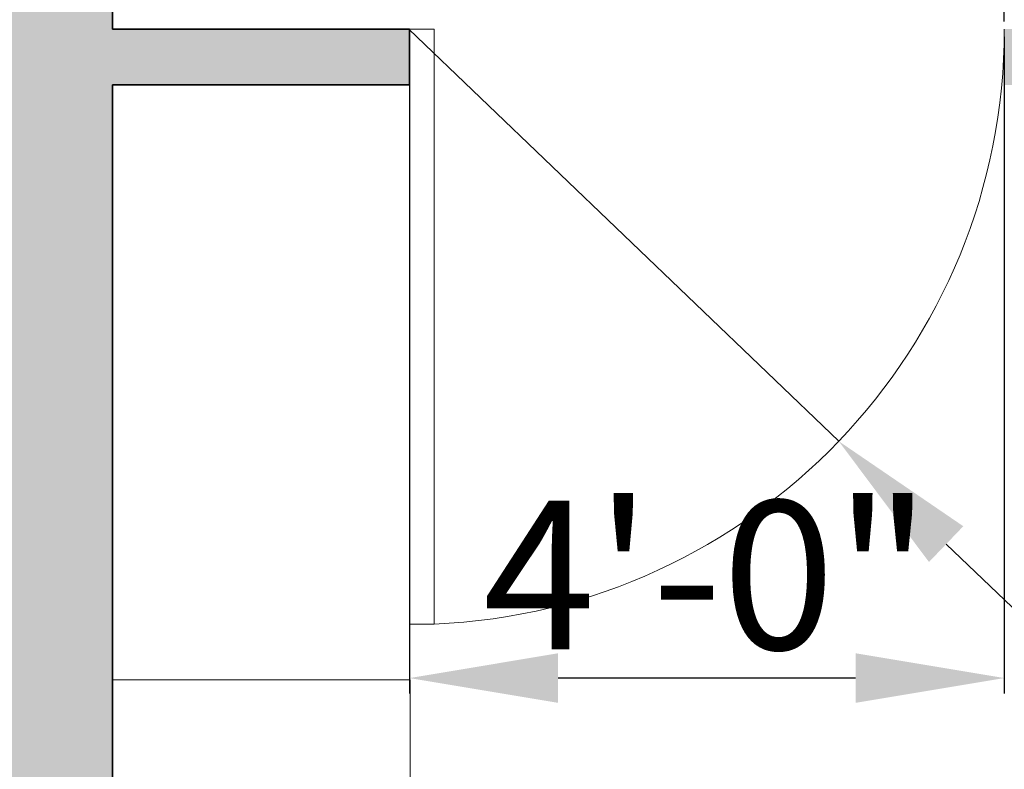
# Model space of a CAD drawing. Units: inches. Extents: x 2083 to 3317, y 1141 to 2115.
# Tile 113 of 256: x 2864 to 2944, y 1361 to 1422. Entities that reach past the tile are written whole.
import ezdxf

# ---------------------------------------------------------------- set-up
doc = ezdxf.new("R2010")
doc.units = ezdxf.units.IN
for name, color, linetype, lineweight in [('A-ANNO-DIMS', 2, 'Continuous', 18), ('A-DOOR', 4, 'Continuous', 18), ('A-FLOR-CASE', 8, 'Continuous', 18), ('A-WALL', 7, 'Continuous', 35)]:
    doc.layers.add(name, color=color, linetype=linetype, lineweight=lineweight)
doc.layers.add('A-WALL-PATT', color=251, linetype='Continuous', lineweight=13, true_color=0x636466)
doc.styles.get("Standard").update_dxf_attribs({"font": 'arial.ttf'})
doc.dimstyles.new('ISO-25', dxfattribs={"dimtxt": 12, "dimasz": 12, "dimexe": 1.25, "dimexo": 0.625, "dimtad": 1, "dimlunit": 3, "dimtxsty": 'Standard', "dimcen": 2.5, "dimadec": 0, "dimazin": 0, "dimtfac": 1, "dimtmove": 0, "dimatfit": 3, "dimfxl": 1, "dimarcsym": 0})

# ---------------------------------------------------------------- blocks, each defined once
blk = doc.blocks.new('CASEWORK-96X24')
for q in [(0, 0), (24, 96)]:
    blk.add_line((0, 96), q)
blk = doc.blocks.new('*D48')
at = {"layer": 'A-ANNO-DIMS', "color": 0, "lineweight": -2, "transparency": 16777216}
for p, q in [((2871.96, 1421.386), (2871.96, 1474.361)), ((2943.91, 1421.386), (2943.91, 1474.361)), ((2883.96, 1473.111), (2931.91, 1473.111))]:
    blk.add_line(p, q, dxfattribs=at)
at = {"layer": 'A-ANNO-DIMS', "color": 0, "transparency": 16777216}
for points in [[(2883.96, 1475.111), (2883.96, 1471.111), (2871.96, 1473.111)], [(2931.91, 1475.111), (2931.91, 1471.111), (2943.91, 1473.111)]]:
    blk.add_solid(points, dxfattribs=at)
at = {"layer": 'Defpoints', "color": 0, "transparency": 16777216}
for p in [(2943.91, 1473.111), (2871.96, 1420.761), (2943.91, 1420.761)]:
    blk.add_point(p, dxfattribs=at)
at = {"layer": 'A-ANNO-DIMS', "color": 0, "transparency": 16777216, "insert": (2907.935, 1479.863), "char_height": 12, "attachment_point": 5}
blk.add_mtext('6\'-0"', dxfattribs=at)
blk = doc.blocks.new('*D59')
at = {"layer": 'A-ANNO-DIMS', "color": 0, "lineweight": -2, "transparency": 16777216}
for p, q in [((2895.91, 1420.136), (2895.91, 1367.161)), ((2943.91, 1420.136), (2943.91, 1367.161)), ((2931.91, 1368.411), (2907.91, 1368.411))]:
    blk.add_line(p, q, dxfattribs=at)
at = {"layer": 'A-ANNO-DIMS', "color": 0, "transparency": 16777216}
for points in [[(2907.91, 1370.411), (2907.91, 1366.411), (2895.91, 1368.411)], [(2931.91, 1370.411), (2931.91, 1366.411), (2943.91, 1368.411)]]:
    blk.add_solid(points, dxfattribs=at)
at = {"layer": 'Defpoints', "color": 0, "transparency": 16777216}
for p in [(2895.91, 1420.761), (2943.91, 1420.761), (2895.91, 1368.411)]:
    blk.add_point(p, dxfattribs=at)
at = {"layer": 'A-ANNO-DIMS', "color": 0, "transparency": 16777216, "insert": (2919.91, 1375.163), "char_height": 12, "attachment_point": 5}
blk.add_mtext('4\'-0"', dxfattribs=at)
blk = doc.blocks.new('*D73')
at = {"layer": 'A-ANNO-DIMS', "color": 0, "lineweight": -2, "transparency": 16777216}
for p, q in [((2895.865, 1420.763), (2930.553, 1387.52)), ((2980.105, 1340.032), (2939.217, 1379.217))]:
    blk.add_line(p, q, dxfattribs=at)
at = {"layer": 'A-ANNO-DIMS', "color": 0, "transparency": 16777216}
blk.add_solid([(2940.601, 1380.661), (2937.833, 1377.773), (2930.553, 1387.52)], dxfattribs=at)
at = {"layer": 'Defpoints', "color": 0, "transparency": 16777216}
for p in [(2895.865, 1420.763), (2930.553, 1387.52)]:
    blk.add_point(p, dxfattribs=at)
at = {"layer": 'A-ANNO-DIMS', "color": 0, "transparency": 16777216, "insert": (2968.665, 1360.348), "char_height": 12, "attachment_point": 5, "rotation": 316.21871}
blk.add_mtext('R4\'-0"', dxfattribs=at)

msp = doc.modelspace()

# ---------------------------------------------------------------- hatches: boundary and pattern name
at = {"layer": 'A-WALL-PATT'}
h = msp.add_hatch(color=256, dxfattribs=at)
h.dxf.hatch_style = 1
h.paths.add_polyline_path([(3126.96, 2020.761), (2748.96, 2020.761), (2604.96, 2020.761), (2226.96, 2020.761), (2226.96, 1702.761), (2466.96, 1702.761), (2466.96, 1582.761), (2418.96, 1582.761), (2418.96, 1477.761), (2226.96, 1477.761), (2226.96, 1263.261), (2544.96, 1263.261), (2544.96, 1411.761), (2604.96, 1411.761), (2685.96, 1411.761), (2685.96, 1420.761), (2604.96, 1420.761), (2604.96, 1573.761), (2604.96, 1702.761), (2604.96, 2011.761), (2748.96, 2011.761), (2748.96, 1702.761), (2862.96, 1702.761), (2862.96, 1621.761), (2871.96, 1621.761), (2871.96, 1702.761), (2883.96, 1702.761), (2883.96, 1706.939, -0.026459), (2883.96, 1711.761), (2757.96, 1711.761), (2757.96, 1807.761), (2787.96, 1807.761), (2787.96, 1812.261), (2757.96, 1812.261), (2757.96, 2011.761), (2877.96, 2011.761), (2877.96, 1812.261), (2847.96, 1812.261), (2847.96, 1807.761), (2889.836, 1807.761), (2889.836, 1812.261), (2882.46, 1812.261), (2882.46, 2011.761), (3117.96, 2011.761), (3117.96, 1812.261), (2937.836, 1812.261), (2937.836, 1807.761), (2995.71, 1807.761), (2995.71, 1796.118), (3000.21, 1796.118), (3000.21, 1807.761), (3117.96, 1807.761), (3117.96, 1711.761), (3000.21, 1711.761), (3000.21, 1760.118), (2998.573, 1760.118, -0.020711), (2995.71, 1760.118), (2995.71, 1711.761), (2931.96, 1711.761), (2931.96, 1702.761), (3126.96, 1702.761)])
h.paths.add_polyline_path([(2471.46, 2011.761), (2471.46, 1810.011), (2462.717, 1810.011), (2462.717, 1805.511), (2505.96, 1805.511), (2505.96, 1810.011), (2475.96, 1810.011), (2475.96, 2011.761), (2595.96, 2011.761), (2595.96, 1810.011), (2565.96, 1810.011), (2565.96, 1805.511), (2595.96, 1805.511), (2595.96, 1711.761), (2235.96, 1711.761), (2235.96, 1805.511), (2353.71, 1805.511), (2353.71, 1796.054), (2358.21, 1796.054), (2358.21, 1805.511), (2414.717, 1805.511), (2414.717, 1810.011), (2235.96, 1810.011), (2235.96, 2011.761)], flags=16)
h.paths.add_polyline_path([(2270.205, 1994.61), (2270.205, 1970.61), (2246.205, 1970.61), (2246.205, 1994.61)], flags=0)
edge = h.paths.add_edge_path(flags=0)
edge.add_ellipse((2332.027, 1899.798), major_axis=(-3.043, 3.043), ratio=0.168252, start_angle=-161.33217, end_angle=-156.30711, ccw=False)
edge.add_ellipse((2333.082, 1898.744), major_axis=(-1.055, 1.055), ratio=0.453532, start_angle=-123.37102, end_angle=-94.15911)
edge = h.paths.add_edge_path(flags=0)
edge.add_ellipse((2332.027, 1968.876), major_axis=(3.043, 3.043), ratio=0.168252, start_angle=18.66783, end_angle=23.69289)
edge.add_spline(control_points=[(2332.926, 1970.691), (2332.227, 1970.336), (2330.894, 1969.659), (2328.413, 1970.932), (2327.204, 1967.749), (2324.71, 1969.956), (2322.533, 1967.012), (2320.013, 1971.296), (2317.68, 1968.158), (2316.041, 1967.102), (2315.427, 1966.81)], knot_values=[0, 0, 0, 0, 2.267059, 4.324559, 6.685584, 8.878641, 11.121502, 14.300359, 17.755284, 19.732645, 19.732645, 19.732645, 19.732645], degree=3, periodic=0)
edge.add_ellipse((2332.027, 1968.876), major_axis=(3.043, 3.043), ratio=0.168252, start_angle=18.66783, end_angle=23.69289, ccw=False)
edge.add_ellipse((2333.082, 1969.931), major_axis=(1.055, 1.055), ratio=0.453532, start_angle=56.62898, end_angle=85.84089, ccw=False)
edge = h.paths.add_edge_path(flags=0)
edge.add_spline(control_points=[(2296.428, 1967.988), (2293.628, 1965.336), (2287.704, 1959.727), (2299.744, 1949.996), (2294.533, 1935.669), (2290.573, 1920.604), (2293.394, 1909.974), (2296.185, 1904.967)], knot_values=[0.099185, 0.099185, 0.099185, 0.099185, 0.345301, 0.619822, 0.982653, 1.386093, 1.810555, 1.810555, 1.810555, 1.810555], degree=3, periodic=0)
edge.add_spline(control_points=[(2296.185, 1904.967), (2297.384, 1902.619), (2298.001, 1901.949), (2298.553, 1901.468)], knot_values=[0.006246, 0.006246, 0.006246, 0.006246, 0.055476, 0.055476, 0.055476, 0.055476], degree=3, periodic=0)
edge.add_spline(control_points=[(2298.553, 1901.468), (2297.259, 1900.923), (2295.225, 1900.232), (2293.06, 1900.614), (2292.101, 1900.788), (2292.09, 1900.791)], knot_values=[0.312835, 0.312835, 0.312835, 0.312835, 0.40178, 0.474987, 0.475903, 0.475903, 0.475903, 0.475903], degree=3, periodic=0)
edge.add_arc((2292.794, 1904.664), 3.937, 215.4209, 259.69818, ccw=False)
edge.add_spline(control_points=[(2289.585, 1902.382), (2289.477, 1902.535), (2289.368, 1902.688), (2289.261, 1902.841)], knot_values=[0.102872, 0.102872, 0.102872, 0.102872, 0.116896, 0.116896, 0.116896, 0.116896], degree=3, periodic=0)
edge.add_spline(control_points=[(2289.261, 1902.841), (2288.687, 1902.55), (2287.64, 1902.02), (2285.881, 1901.874), (2283.853, 1901.504), (2281.72, 1899.711), (2278.467, 1899.493), (2276.157, 1901.883), (2272.259, 1899.804), (2267.778, 1901.843), (2262.244, 1900.184), (2257.415, 1901.782), (2254.318, 1900.726), (2253.178, 1900.337)], knot_values=[0, 0, 0, 0, 1.907977, 3.477176, 5.261074, 7.972851, 11.680248, 13.717921, 16.939592, 22.789562, 27.502503, 33.595215, 37.145618, 37.145618, 37.145618, 37.145618], degree=3, periodic=0)
edge.add_line((2253.178, 1900.337), (2250.244, 1902.841))
edge.add_line((2250.244, 1902.841), (2250.244, 1965.833))
edge.add_line((2250.244, 1965.833), (2253.178, 1968.337))
edge.add_spline(control_points=[(2253.178, 1968.337), (2254.318, 1967.948), (2257.415, 1966.892), (2262.244, 1968.49), (2267.778, 1966.831), (2271.527, 1968.537), (2273.876, 1967.828), (2274.207, 1967.728)], knot_values=[0, 0, 0, 0, 0.09018, 0.244935, 0.364644, 0.513233, 0.537855, 0.537855, 0.537855, 0.537855], degree=3, periodic=0)
edge.add_arc((2274.353, 1963.793), 3.937, 72.05113, 92.12795, ccw=False)
edge.add_arc((2281.297, 1985.23), 18.596, 252.05113, 288.56572)
edge.add_arc((2292.317, 1956.029), 12.646, 71.02679, 113.77822, ccw=False)
edge = h.paths.add_edge_path(flags=0)
edge.add_spline(control_points=[(2274.899, 1951.856), (2275.066, 1951.617), (2275.233, 1951.377), (2275.398, 1951.136)], knot_values=[1.409916, 1.409916, 1.409916, 1.409916, 1.43159, 1.43159, 1.43159, 1.43159], degree=3, periodic=0)
edge.add_spline(control_points=[(2275.398, 1951.136), (2275.792, 1950.562), (2276.179, 1949.984), (2276.546, 1949.397)], knot_values=[1.358238, 1.358238, 1.358238, 1.358238, 1.409916, 1.409916, 1.409916, 1.409916], degree=3, periodic=0)
edge.add_line((2276.546, 1949.397), (2277.437, 1947.862))
edge.add_spline(control_points=[(2277.437, 1947.862), (2276.304, 1945.673), (2274.64, 1942.427), (2274.632, 1938.094), (2272.799, 1930.852), (2274.356, 1943.897), (2275.948, 1947.923), (2276.546, 1949.397)], knot_values=[0.005632, 0.005632, 0.005632, 0.005632, 0.186014, 0.266002, 0.357087, 0.59639, 0.739732, 0.739732, 0.739732, 0.739732], degree=3, periodic=0)
edge.add_spline(control_points=[(2276.546, 1949.397), (2276.179, 1949.984), (2275.792, 1950.562), (2275.398, 1951.136)], knot_values=[1.358238, 1.358238, 1.358238, 1.358238, 1.409916, 1.409916, 1.409916, 1.409916], degree=3, periodic=0)
edge.add_spline(control_points=[(2275.398, 1951.136), (2274.943, 1950.08), (2274.208, 1948.025), (2273.935, 1944.851), (2272.469, 1937.627), (2273.466, 1945.696), (2274.701, 1951.059), (2274.899, 1951.856)], knot_values=[0.104364, 0.104364, 0.104364, 0.104364, 0.189636, 0.269624, 0.36071, 0.600013, 0.644622, 0.644622, 0.644622, 0.644622], degree=3, periodic=0)
h.paths.add_polyline_path([(2269.168, 1963.128, -0.357527), (2268.171, 1960.976, -0.092561), (2268.171, 1939.436, -0.357527), (2269.168, 1937.285, -0.357527), (2267.016, 1938.282, -0.164785), (2254.686, 1938.282, -0.357527), (2252.534, 1937.285, -0.357527), (2253.531, 1939.436, -0.092561), (2253.531, 1960.976, -0.357527), (2252.534, 1963.128, -0.357527), (2254.686, 1962.131, -0.164785), (2267.016, 1962.131, -0.357527)], flags=0)
h.paths.add_polyline_path([(2248.874, 1967.802), (2248.874, 1957.028), (2249.458, 1957.028), (2249.458, 1911.647), (2248.874, 1911.647), (2248.874, 1900.873), (2246.512, 1900.873, 0.197327), (2244.15, 1902.457), (2244.15, 1966.218, 0.197327), (2246.512, 1967.802)], flags=0)
h.paths.add_polyline_path([(2269.168, 1931.389, -0.357527), (2268.171, 1929.238, -0.092561), (2268.171, 1907.698, -0.357527), (2269.168, 1905.547, -0.357527), (2267.016, 1906.544, -0.164785), (2254.686, 1906.544, -0.357527), (2252.534, 1905.547, -0.357527), (2253.531, 1907.698, -0.092561), (2253.531, 1929.238, -0.357527), (2252.534, 1931.389, -0.357527), (2254.686, 1930.392, -0.164785), (2267.016, 1930.392, -0.357527)], flags=0)
edge = h.paths.add_edge_path(flags=0)
edge.add_spline(control_points=[(2276.197, 1906.724), (2276.168, 1909.029), (2276.114, 1913.372), (2270.598, 1924.925), (2273.905, 1919.013), (2275.922, 1916.262), (2275.475, 1912.402), (2277.258, 1910.381), (2276.696, 1908.225), (2276.646, 1906.813), (2276.618, 1906.008)], knot_values=[0, 0, 0, 0, 8.61026, 16.221274, 18.843057, 23.804898, 27.440828, 29.356102, 31.203478, 33.650687, 33.650687, 33.650687, 33.650687], degree=3, periodic=0)
edge.add_spline(control_points=[(2276.618, 1906.008), (2276.623, 1905.624), (2276.498, 1904.629), (2275.442, 1903.855), (2274.937, 1903.08), (2274.859, 1902.841)], knot_values=[0.156488, 0.156488, 0.156488, 0.156488, 0.184398, 0.231376, 0.250598, 0.250598, 0.250598, 0.250598], degree=3, periodic=0)
edge.add_line((2274.859, 1902.841), (2276.506, 1902.841))
edge.add_spline(control_points=[(2276.506, 1902.841), (2276.788, 1903.085), (2277.665, 1904.125), (2278.25, 1904.341), (2277.654, 1908.527), (2278.156, 1906.228), (2278.1, 1905.286), (2278.847, 1904.069), (2277.857, 1903.415), (2277.874, 1902.991), (2277.904, 1902.841)], knot_values=[0.059574, 0.059574, 0.059574, 0.059574, 0.080753, 0.103741, 0.16972, 0.176036, 0.207137, 0.240474, 0.262341, 0.27366, 0.27366, 0.27366, 0.27366], degree=3, periodic=0)
edge.add_line((2277.904, 1902.841), (2280.03, 1902.841))
edge.add_spline(control_points=[(2280.03, 1902.841), (2279.888, 1903.088), (2279.499, 1903.982), (2280.152, 1905.939), (2278.104, 1909.658), (2279.762, 1907.185), (2280.328, 1904.875), (2280.485, 1903.49), (2281.463, 1903.249), (2281.758, 1902.936), (2281.834, 1902.841)], knot_values=[0.013856, 0.013856, 0.013856, 0.013856, 0.034874, 0.088867, 0.107879, 0.126738, 0.158714, 0.193757, 0.217487, 0.226722, 0.226722, 0.226722, 0.226722], degree=3, periodic=0)
edge.add_spline(control_points=[(2281.834, 1902.841), (2281.788, 1902.827), (2281.647, 1902.783), (2281.396, 1902.859), (2281.088, 1902.985), (2280.721, 1903.061), (2280.333, 1903.026), (2280.125, 1902.899), (2280.03, 1902.841)], knot_values=[0, 0, 0, 0, 0.14413, 0.435517, 0.749276, 1.153046, 1.548371, 1.878348, 1.878348, 1.878348, 1.878348], degree=3, periodic=0)
edge.add_line((2280.03, 1902.841), (2277.904, 1902.841))
edge.add_spline(control_points=[(2277.904, 1902.841), (2277.893, 1902.796), (2277.865, 1902.68), (2277.607, 1902.687), (2277.274, 1902.801), (2276.838, 1902.62), (2276.584, 1902.789), (2276.506, 1902.841)], knot_values=[0, 0, 0, 0, 0.127189, 0.326199, 0.628009, 1.24357, 1.515331, 1.515331, 1.515331, 1.515331], degree=3, periodic=0)
edge.add_line((2276.506, 1902.841), (2274.859, 1902.841))
edge.add_spline(control_points=[(2274.859, 1902.841), (2274.814, 1902.899), (2274.725, 1903.013), (2274.493, 1903.119), (2274.244, 1902.961), (2273.937, 1903.185), (2273.614, 1902.983), (2273.408, 1902.883), (2273.322, 1902.841)], knot_values=[0, 0, 0, 0, 0.21843, 0.436957, 0.687977, 0.990379, 1.398396, 1.69185, 1.69185, 1.69185, 1.69185], degree=3, periodic=0)
edge.add_spline(control_points=[(2273.322, 1902.841), (2273.617, 1903.446), (2274.274, 1904.538), (2276.027, 1904.574), (2276.207, 1906.584), (2276.197, 1906.724)], knot_values=[0.012227, 0.012227, 0.012227, 0.012227, 0.059472, 0.106218, 0.134458, 0.134458, 0.134458, 0.134458], degree=3, periodic=0)
h.paths.add_polyline_path([(2270.776, 1897.79), (2270.776, 1873.79), (2246.776, 1873.79), (2246.776, 1897.79)], flags=0)
h.paths.add_polyline_path([(2353.71, 1760.005), (2353.71, 1760.054), (2358.21, 1760.054, -0.033729)], flags=0)
h.paths.add_polyline_path([(2321.819, 1737.529), (2341.995, 1737.529, -0.414214), (2343.203, 1736.321), (2343.203, 1721.021, -0.414214), (2341.995, 1719.813), (2321.819, 1719.813, -0.414214), (2320.611, 1721.021), (2320.611, 1736.321, -0.414214)], flags=0)
h.paths.add_polyline_path([(2324.235, 1736.321), (2339.579, 1736.321, -0.414214), (2341.995, 1733.905), (2341.995, 1725.45, -0.414214), (2339.579, 1723.034), (2333.681, 1723.034), (2333.845, 1722.045, -0.870646), (2335.425, 1721.826, -0.767327), (2333.923, 1721.423), (2331.291, 1721.423, -0.767327), (2329.788, 1721.826, -0.870646), (2331.368, 1722.045), (2331.533, 1723.034), (2324.235, 1723.034, -0.414214), (2321.819, 1725.45), (2321.819, 1733.905, -0.414214)], flags=0)
h.paths.add_polyline_path([(2570.484, 1928.615), (2589.684, 1928.615), (2590.169, 1928.615), (2590.169, 1904.993), (2570.484, 1904.993)], flags=0)
h.paths.add_polyline_path([(2574.447, 1927.264, -1), (2572.829, 1927.264, -1)], flags=0)
h.paths.add_polyline_path([(2573.09, 1926.941), (2573.925, 1927.776), (2574.148, 1927.553), (2573.313, 1926.718)], flags=0)
h.paths.add_polyline_path([(2578.779, 1919.73, -1), (2571.592, 1919.73, -1)], flags=0)
h.paths.add_polyline_path([(2578.385, 1919.73, -1), (2571.985, 1919.73, -1)], flags=0)
h.paths.add_polyline_path([(2331.596, 1729.476, -1), (2333.618, 1729.476, -1)], flags=0)
h.paths.add_polyline_path([(2578.034, 1927.264, -1), (2576.416, 1927.264, -1)], flags=0)
h.paths.add_polyline_path([(2576.689, 1927.531), (2576.912, 1927.754), (2577.747, 1926.919), (2577.524, 1926.696)], flags=0)
h.paths.add_polyline_path([(2578.139, 1909.86, -1), (2572.232, 1909.86, -1)], flags=0)
h.paths.add_polyline_path([(2577.745, 1909.86, -1), (2572.625, 1909.86, -1)], flags=0)
h.paths.add_polyline_path([(2583.798, 1927.264, -1), (2582.179, 1927.264, -1)], flags=0)
h.paths.add_polyline_path([(2582.719, 1927.754), (2583.554, 1926.919), (2583.331, 1926.696), (2582.496, 1927.531)], flags=0)
h.paths.add_polyline_path([(2582.496, 1927.531), (2582.719, 1927.754), (2583.554, 1926.919), (2583.331, 1926.696)], flags=0)
h.paths.add_polyline_path([(2587.739, 1920.53, -1), (2581.832, 1920.53, -1)], flags=0)
h.paths.add_polyline_path([(2587.345, 1920.53, -1), (2582.225, 1920.53, -1)], flags=0)
h.paths.add_polyline_path([(2587.385, 1927.264, -1), (2585.766, 1927.264, -1)], flags=0)
h.paths.add_polyline_path([(2586.082, 1926.98), (2586.917, 1927.815), (2587.14, 1927.593), (2586.305, 1926.758)], flags=0)
h.paths.add_polyline_path([(2588.379, 1910.66, -1), (2581.192, 1910.66, -1)], flags=0)
h.paths.add_polyline_path([(2587.985, 1910.66, -1), (2581.585, 1910.66, -1)], flags=0)
h.paths.add_polyline_path([(2417.168, 1729.478), (2437.344, 1729.478, -0.414214), (2438.552, 1728.27), (2438.552, 1712.969, -0.414214), (2437.344, 1711.761), (2417.168, 1711.761, -0.414214), (2415.96, 1712.969), (2415.96, 1728.27, -0.414214)], flags=0)
h.paths.add_polyline_path([(2419.584, 1728.27), (2434.928, 1728.27, -0.414214), (2437.344, 1725.854), (2437.344, 1717.398, -0.414214), (2434.928, 1714.983), (2429.029, 1714.983), (2429.194, 1713.994, -0.870646), (2430.774, 1713.775, -0.767327), (2429.271, 1713.372), (2426.64, 1713.372, -0.767327), (2425.137, 1713.775, -0.870646), (2426.717, 1713.994), (2426.882, 1714.983), (2419.584, 1714.983, -0.414214), (2417.168, 1717.398), (2417.168, 1725.854, -0.414214)], flags=0)
h.paths.add_polyline_path([(2419.584, 1728.27), (2434.928, 1728.27, -0.414214), (2437.344, 1725.854), (2437.344, 1717.398, -0.414214), (2434.928, 1714.983), (2429.029, 1714.983), (2428.358, 1719.009), (2427.553, 1719.009), (2426.882, 1714.983), (2419.584, 1714.983, -0.414214), (2417.168, 1717.398), (2417.168, 1725.854, -0.414214)], flags=0)
h.paths.add_polyline_path([(2426.944, 1721.425, -1), (2428.967, 1721.425, -1)], flags=0)
h.paths.add_polyline_path([(2475.96, 1702.761), (2595.96, 1702.761), (2595.96, 1582.761), (2475.96, 1582.761)], flags=16)
h.paths.add_polyline_path([(2427.96, 1573.761), (2595.96, 1573.761), (2595.96, 1468.761), (2595.96, 1420.761), (2384.46, 1420.761), (2384.46, 1468.761), (2427.96, 1468.761)], flags=16)
h.paths.add_polyline_path([(2379.96, 1468.761), (2379.96, 1420.761), (2235.96, 1420.761), (2235.96, 1468.761)], flags=16)
h.paths.add_polyline_path([(2317.816, 1466.696), (2337.992, 1466.696, -0.414214), (2339.2, 1465.488), (2339.2, 1450.187, -0.414214), (2337.992, 1448.979), (2317.816, 1448.979, -0.414214), (2316.608, 1450.187), (2316.608, 1465.488, -0.414214)], flags=0)
h.paths.add_polyline_path([(2320.232, 1465.488), (2335.576, 1465.488, -0.414214), (2337.992, 1463.072), (2337.992, 1454.616, -0.414214), (2335.576, 1452.2), (2329.677, 1452.2), (2329.842, 1451.212, -0.870646), (2331.422, 1450.992, -0.767327), (2329.92, 1450.59), (2327.288, 1450.59, -0.767327), (2325.785, 1450.992, -0.870646), (2327.365, 1451.212), (2327.53, 1452.2), (2320.232, 1452.2, -0.414214), (2317.816, 1454.616), (2317.816, 1463.072, -0.414214)], flags=0)
h.paths.add_polyline_path([(2320.232, 1465.488), (2335.576, 1465.488, -0.414214), (2337.992, 1463.072), (2337.992, 1454.616, -0.414214), (2335.576, 1452.2), (2329.677, 1452.2), (2329.006, 1456.227), (2328.201, 1456.227), (2327.53, 1452.2), (2320.232, 1452.2, -0.414214), (2317.816, 1454.616), (2317.816, 1463.072, -0.414214)], flags=0)
h.paths.add_polyline_path([(2327.593, 1458.643, -1), (2329.615, 1458.643, -1)], flags=0)
h.paths.add_polyline_path([(2244.412, 1433.34), (2241.921, 1433.34, -0.414214), (2240.018, 1435.244), (2240.018, 1440.953, -0.414211), (2241.921, 1442.856), (2244.412, 1442.856, -1.976472)], flags=0)
h.paths.add_polyline_path([(2245.357, 1434.398, -0.414214), (2245.357, 1441.799, -2.144098)], flags=0)
h.paths.add_polyline_path([(2535.96, 1416.261), (2535.96, 1272.261), (2235.96, 1272.261), (2235.96, 1416.261)], flags=16)
h.paths.add_polyline_path([(2260.12, 1384.293), (2260.12, 1362.039), (2237.865, 1362.039), (2237.865, 1384.293)], flags=0)
edge = h.paths.add_edge_path(flags=0)
edge.add_line((2318.252, 1362.093), (2318.146, 1362.001))
edge.add_ellipse((2317.445, 1360.431), major_axis=(2.822, 2.822), ratio=0.168252, start_angle=18.66783, end_angle=20.94813, ccw=False)
edge.add_ellipse((2318.423, 1361.409), major_axis=(0.978, 0.978), ratio=0.453532, start_angle=56.62898, end_angle=70.2262, ccw=False)
edge = h.paths.add_edge_path(flags=0)
edge.add_line((2319.107, 1295.571), (2319.015, 1295.677))
edge.add_ellipse((2317.445, 1296.378), major_axis=(-2.822, 2.822), ratio=0.168252, start_angle=-161.33217, end_angle=-159.05187, ccw=False)
edge.add_ellipse((2318.423, 1295.4), major_axis=(-0.978, 0.978), ratio=0.453532, start_angle=-123.37102, end_angle=-109.7738)
edge = h.paths.add_edge_path(flags=0)
edge.add_spline(control_points=[(2284.21, 1301.17), (2284.581, 1300.445), (2284.891, 1299.892), (2285.16, 1299.461)], knot_values=[0.039066, 0.039066, 0.039066, 0.039066, 0.055476, 0.055476, 0.055476, 0.055476], degree=3, periodic=0)
edge.add_line((2285.16, 1299.461), (2284.21, 1301.17))
edge = h.paths.add_edge_path(flags=0)
edge.add_line((2280.412, 1297.298), (2283.37, 1297.036))
edge.add_line((2283.37, 1297.036), (2286.406, 1297.926))
edge.add_spline(control_points=[(2286.406, 1297.926), (2285.305, 1297.463), (2284.345, 1297.129), (2283.37, 1297.036)], knot_values=[0.394369, 0.394369, 0.394369, 0.394369, 0.475903, 0.475903, 0.475903, 0.475903], degree=3, periodic=0)
edge.add_spline(control_points=[(2283.37, 1297.036), (2283.281, 1297.028), (2282.316, 1296.957), (2281.313, 1297.134), (2280.423, 1297.296), (2280.412, 1297.298)], knot_values=[0.312835, 0.312835, 0.312835, 0.312835, 0.320246, 0.393453, 0.394369, 0.394369, 0.394369, 0.394369], degree=3, periodic=0)
edge = h.paths.add_edge_path(flags=0)
edge.add_line((2284.436, 1359.607), (2280.446, 1355.328))
edge.add_line((2280.446, 1355.328), (2279.58, 1351.018))
edge.add_line((2279.58, 1351.018), (2282.413, 1346.58))
edge.add_spline(control_points=[(2282.413, 1346.58), (2283.153, 1345.589), (2284.253, 1344.029), (2284.801, 1342.387), (2284.935, 1341.806)], knot_values=[1.240098, 1.240098, 1.240098, 1.240098, 1.332892, 1.382712, 1.382712, 1.382712, 1.382712], degree=3, periodic=0)
edge.add_spline(control_points=[(2284.935, 1341.806), (2285.319, 1340.141), (2285.233, 1338.409), (2284.91, 1336.654)], knot_values=[1.097484, 1.097484, 1.097484, 1.097484, 1.240098, 1.240098, 1.240098, 1.240098], degree=3, periodic=0)
edge.add_spline(control_points=[(2284.91, 1336.654), (2284.587, 1334.899), (2284.027, 1333.12), (2283.463, 1331.361)], knot_values=[0.95487, 0.95487, 0.95487, 0.95487, 1.097484, 1.097484, 1.097484, 1.097484], degree=3, periodic=0)
edge.add_line((2283.463, 1331.361), (2281.89, 1326.153))
edge.add_line((2281.89, 1326.153), (2280.756, 1321.056))
edge.add_line((2280.756, 1321.056), (2280.299, 1316.002))
edge.add_line((2280.299, 1316.002), (2280.716, 1310.95))
edge.add_line((2280.716, 1310.95), (2282.028, 1305.972))
edge.add_line((2282.028, 1305.972), (2284.21, 1301.17))
edge.add_spline(control_points=[(2284.21, 1301.17), (2283.341, 1302.73), (2282.612, 1304.336), (2282.028, 1305.972)], knot_values=[0.099185, 0.099185, 0.099185, 0.099185, 0.241799, 0.241799, 0.241799, 0.241799], degree=3, periodic=0)
edge.add_spline(control_points=[(2282.028, 1305.972), (2281.444, 1307.608), (2281.005, 1309.273), (2280.716, 1310.95)], knot_values=[0.241799, 0.241799, 0.241799, 0.241799, 0.384413, 0.384413, 0.384413, 0.384413], degree=3, periodic=0)
edge.add_spline(control_points=[(2280.716, 1310.95), (2280.433, 1312.588), (2280.289, 1314.277), (2280.299, 1315.962), (2280.299, 1316.002)], knot_values=[0.384413, 0.384413, 0.384413, 0.384413, 0.523647, 0.527028, 0.527028, 0.527028, 0.527028], degree=3, periodic=0)
edge.add_spline(control_points=[(2280.299, 1316.002), (2280.312, 1317.687), (2280.478, 1319.368), (2280.756, 1321.056)], knot_values=[0.527028, 0.527028, 0.527028, 0.527028, 0.669642, 0.669642, 0.669642, 0.669642], degree=3, periodic=0)
edge.add_spline(control_points=[(2280.756, 1321.056), (2281.035, 1322.744), (2281.426, 1324.44), (2281.89, 1326.153)], knot_values=[0.669642, 0.669642, 0.669642, 0.669642, 0.812256, 0.812256, 0.812256, 0.812256], degree=3, periodic=0)
edge.add_spline(control_points=[(2281.89, 1326.153), (2282.264, 1327.533), (2282.788, 1329.262), (2283.353, 1331.018), (2283.463, 1331.361)], knot_values=[0.812256, 0.812256, 0.812256, 0.812256, 0.927087, 0.95487, 0.95487, 0.95487, 0.95487], degree=3, periodic=0)
edge.add_line((2283.463, 1331.361), (2284.91, 1336.654))
edge.add_line((2284.91, 1336.654), (2284.935, 1341.806))
edge.add_line((2284.935, 1341.806), (2282.413, 1346.58))
edge.add_spline(control_points=[(2282.413, 1346.58), (2281.275, 1348.104), (2280.078, 1349.57), (2279.58, 1351.018)], knot_values=[1.382712, 1.382712, 1.382712, 1.382712, 1.525326, 1.525326, 1.525326, 1.525326], degree=3, periodic=0)
edge.add_spline(control_points=[(2279.58, 1351.018), (2279.443, 1351.415), (2279.136, 1352.857), (2279.735, 1354.29), (2280.446, 1355.328)], knot_values=[1.525326, 1.525326, 1.525326, 1.525326, 1.564439, 1.667941, 1.667941, 1.667941, 1.667941], degree=3, periodic=0)
edge.add_spline(control_points=[(2280.446, 1355.328), (2281.426, 1356.758), (2282.931, 1358.183), (2284.436, 1359.607)], knot_values=[1.667941, 1.667941, 1.667941, 1.667941, 1.810555, 1.810555, 1.810555, 1.810555], degree=3, periodic=0)
edge.add_arc((2280.623, 1348.518), 11.726, 71.02679, 113.77822)
edge.add_arc((2270.405, 1375.595), 17.244, 252.05113, 288.56572, ccw=False)
edge.add_arc((2263.966, 1355.718), 3.651, 72.05113, 92.12795)
edge.add_arc((2263.966, 1355.718), 3.651, 92.12795, 177.98513)
edge.add_spline(control_points=[(2260.318, 1355.846), (2260.26, 1354.221), (2260.551, 1350.187), (2262.999, 1346.766), (2264.473, 1344.649)], knot_values=[1.43159, 1.43159, 1.43159, 1.43159, 1.564144, 1.770695, 1.770695, 1.770695, 1.770695], degree=3, periodic=0)
edge.add_line((2264.473, 1344.649), (2264.936, 1343.983))
edge.add_spline(control_points=[(2263.801, 1340.248), (2263.843, 1340.514), (2264.067, 1341.756), (2264.513, 1343.002), (2264.935, 1343.981)], knot_values=[0.53657, 0.53657, 0.53657, 0.53657, 0.559349, 0.644622, 0.644622, 0.644622, 0.644622], degree=3, periodic=0)
edge.add_spline(control_points=[(2264.935, 1343.981), (2265.118, 1343.715), (2265.299, 1343.448), (2265.477, 1343.179)], knot_values=[1.384077, 1.384077, 1.384077, 1.384077, 1.409916, 1.409916, 1.409916, 1.409916], degree=3, periodic=0)
edge.add_spline(control_points=[(2265.477, 1343.179), (2265.655, 1342.911), (2265.829, 1342.641), (2265.999, 1342.369)], knot_values=[1.358238, 1.358238, 1.358238, 1.358238, 1.384077, 1.384077, 1.384077, 1.384077], degree=3, periodic=0)
edge.add_line((2265.999, 1342.369), (2266.826, 1340.946))
edge.add_spline(control_points=[(2266.826, 1340.946), (2268.894, 1337.09), (2271.398, 1325.843), (2270.516, 1310.569), (2275.919, 1301.861), (2277.79, 1299.199)], knot_values=[0.116896, 0.116896, 0.116896, 0.116896, 0.472987, 1.050969, 1.313793, 1.313793, 1.313793, 1.313793], degree=3, periodic=0)
edge.add_spline(control_points=[(2277.79, 1299.199), (2277.839, 1299.128), (2277.889, 1299.057), (2277.94, 1298.987)], knot_values=[0.109884, 0.109884, 0.109884, 0.109884, 0.116896, 0.116896, 0.116896, 0.116896], degree=3, periodic=0)
edge.add_line((2277.94, 1298.987), (2277.789, 1299.199))
edge.add_spline(control_points=[(2277.789, 1299.199), (2277.257, 1298.929), (2276.286, 1298.438), (2275.039, 1298.334), (2274.383, 1298.239), (2274.215, 1298.209)], knot_values=[33.12187, 33.12187, 33.12187, 33.12187, 35.029056, 36.598255, 37.144827, 37.144827, 37.144827, 37.144827], degree=3, periodic=0)
edge.add_line((2274.215, 1298.209), (2273.073, 1297.893))
edge.add_spline(control_points=[(2273.073, 1297.893), (2272.323, 1297.58), (2271.039, 1296.511), (2269.248, 1296.226), (2268.423, 1296.375)], knot_values=[26.532584, 26.532584, 26.532584, 26.532584, 29.198919, 31.839101, 31.839101, 31.839101, 31.839101], degree=3, periodic=0)
edge.add_line((2268.423, 1296.375), (2263.879, 1297.458))
edge.add_spline(control_points=[(2263.879, 1297.458), (2263.556, 1297.359), (2261.86, 1296.839), (2260.239, 1297.282), (2258.933, 1297.516)], knot_values=[15.919551, 15.919551, 15.919551, 15.919551, 16.939592, 21.226067, 21.226067, 21.226067, 21.226067], degree=3, periodic=0)
edge.add_line((2258.933, 1297.516), (2254.055, 1297.329))
edge.add_spline(control_points=[(2254.055, 1297.329), (2253.756, 1297.296), (2252.114, 1297.165), (2250.462, 1297.544), (2249.13, 1297.668)], knot_values=[5.306517, 5.306517, 5.306517, 5.306517, 6.276435, 10.613034, 10.613034, 10.613034, 10.613034], degree=3, periodic=0)
edge.add_line((2249.13, 1297.668), (2244.332, 1296.878))
edge.add_line((2244.332, 1296.878), (2241.611, 1299.199))
edge.add_line((2241.611, 1299.199), (2241.611, 1357.609))
edge.add_line((2241.611, 1357.609), (2244.332, 1359.931))
edge.add_line((2244.332, 1359.931), (2252.729, 1359.543))
edge.add_spline(control_points=[(2252.729, 1359.543), (2252.871, 1359.546), (2253.306, 1359.548), (2253.74, 1359.514), (2254.032, 1359.482)], knot_values=[0.233291, 0.233291, 0.233291, 0.233291, 0.244935, 0.268927, 0.268927, 0.268927, 0.268927], degree=3, periodic=0)
edge.add_line((2254.032, 1359.482), (2259.587, 1359.416))
edge.add_spline(control_points=[(2259.587, 1359.416), (2260.677, 1359.629), (2262.073, 1359.897), (2263.524, 1359.459), (2263.83, 1359.366)], knot_values=[0.422516, 0.422516, 0.422516, 0.422516, 0.513233, 0.537855, 0.537855, 0.537855, 0.537855], degree=3, periodic=0)
edge.add_arc((2263.966, 1355.718), 3.651, 72.05113, 92.12795, ccw=False)
edge.add_arc((2270.405, 1375.595), 17.244, 252.05113, 288.56572)
edge.add_arc((2280.623, 1348.518), 11.726, 71.02679, 113.77822, ccw=False)
h.paths.add_polyline_path([(2240.341, 1359.435), (2240.341, 1349.444), (2240.882, 1349.444), (2240.882, 1307.365), (2240.341, 1307.365), (2240.341, 1297.374), (2238.15, 1297.374, 0.197327), (2235.96, 1298.843), (2235.96, 1357.966, 0.197327), (2238.15, 1359.435)], flags=0)
h.paths.add_polyline_path([(2259.158, 1355.101, -0.357527), (2258.233, 1353.106, -0.092561), (2258.233, 1333.133, -0.357527), (2259.158, 1331.138, -0.357527), (2257.163, 1332.062, -0.164785), (2245.729, 1332.062, -0.357527), (2243.735, 1331.138, -0.357527), (2244.659, 1333.133, -0.092561), (2244.659, 1353.106, -0.357527), (2243.735, 1355.101, -0.357527), (2245.729, 1354.176, -0.164785), (2257.163, 1354.176, -0.357527)], flags=0)
edge = h.paths.add_edge_path(flags=0)
edge.add_line((2265.999, 1342.369), (2266.826, 1340.946))
edge.add_line((2266.826, 1340.946), (2265.308, 1337.814))
edge.add_line((2265.308, 1337.814), (2264.358, 1334.653))
edge.add_line((2264.358, 1334.653), (2264.262, 1333.8))
edge.add_spline(control_points=[(2264.262, 1333.8), (2264.208, 1333.187), (2264.162, 1332.366), (2264.007, 1331.414), (2263.969, 1331.202)], knot_values=[0.464444, 0.464444, 0.464444, 0.464444, 0.516691, 0.531608, 0.531608, 0.531608, 0.531608], degree=3, periodic=0)
edge.add_spline(control_points=[(2263.969, 1331.202), (2263.775, 1330.119), (2263.424, 1328.791), (2263.257, 1328.531), (2263.234, 1328.515)], knot_values=[0.372682, 0.372682, 0.372682, 0.372682, 0.44885, 0.464444, 0.464444, 0.464444, 0.464444], degree=3, periodic=0)
edge.add_spline(control_points=[(2263.234, 1328.515), (2263.096, 1328.42), (2263.131, 1329.301), (2263.275, 1330.616)], knot_values=[0.280919, 0.280919, 0.280919, 0.280919, 0.372682, 0.372682, 0.372682, 0.372682], degree=3, periodic=0)
edge.add_spline(control_points=[(2263.275, 1330.616), (2263.419, 1331.93), (2263.672, 1333.677), (2263.97, 1335.315)], knot_values=[0.189157, 0.189157, 0.189157, 0.189157, 0.280919, 0.280919, 0.280919, 0.280919], degree=3, periodic=0)
edge.add_spline(control_points=[(2263.97, 1335.315), (2264.1, 1336.032), (2264.419, 1337.622), (2264.755, 1338.864), (2264.947, 1339.491)], knot_values=[0.097394, 0.097394, 0.097394, 0.097394, 0.137578, 0.189157, 0.189157, 0.189157, 0.189157], degree=3, periodic=0)
edge.add_spline(control_points=[(2264.947, 1339.491), (2265.29, 1340.606), (2265.644, 1341.494), (2265.999, 1342.369)], knot_values=[0.005632, 0.005632, 0.005632, 0.005632, 0.097394, 0.097394, 0.097394, 0.097394], degree=3, periodic=0)
h.paths.add_polyline_path([(2259.158, 1325.671, -0.357527), (2258.233, 1323.676, -0.092561), (2258.233, 1303.703, -0.357527), (2259.158, 1301.708, -0.357527), (2257.163, 1302.633, -0.164785), (2245.729, 1302.633, -0.357527), (2243.735, 1301.708, -0.357527), (2244.659, 1303.703, -0.092561), (2244.659, 1323.676, -0.357527), (2243.735, 1325.671, -0.357527), (2245.729, 1324.747, -0.164785), (2257.163, 1324.747, -0.357527)], flags=0)
edge = h.paths.add_edge_path(flags=0)
edge.add_spline(control_points=[(2261.709, 1317.311), (2261.679, 1317.418), (2261.762, 1317.389), (2262.491, 1316.09), (2262.962, 1315.301)], knot_values=[14.955861, 14.955861, 14.955861, 14.955861, 16.221274, 18.694826, 18.694826, 18.694826, 18.694826], degree=3, periodic=0)
edge.add_spline(control_points=[(2262.962, 1315.301), (2262.99, 1315.254), (2263.702, 1314.067), (2264.349, 1313.127), (2264.73, 1312.164)], knot_values=[18.694826, 18.694826, 18.694826, 18.694826, 18.843057, 22.433791, 22.433791, 22.433791, 22.433791], degree=3, periodic=0)
edge.add_spline(control_points=[(2264.73, 1312.164), (2264.876, 1311.796), (2265.177, 1310.77), (2265.143, 1309.559), (2265.248, 1308.824)], knot_values=[22.433791, 22.433791, 22.433791, 22.433791, 23.804898, 26.172756, 26.172756, 26.172756, 26.172756], degree=3, periodic=0)
edge.add_line((2265.248, 1308.824), (2265.851, 1307.172))
edge.add_spline(control_points=[(2265.851, 1307.172), (2266.065, 1306.822), (2266.384, 1306.332), (2266.424, 1305.781), (2266.42, 1305.611)], knot_values=[28.062562, 28.062562, 28.062562, 28.062562, 29.356102, 29.911721, 29.911721, 29.911721, 29.911721], degree=3, periodic=0)
edge.add_spline(control_points=[(2266.42, 1305.611), (2266.416, 1305.433), (2266.394, 1305.25), (2266.365, 1305.066)], knot_values=[29.911721, 29.911721, 29.911721, 29.911721, 30.497837, 30.497837, 30.497837, 30.497837], degree=3, periodic=0)
edge.add_line((2266.365, 1305.066), (2266.066, 1302.136))
edge.add_spline(control_points=[(2266.066, 1302.136), (2266.071, 1301.78), (2265.998, 1301.2), (2265.663, 1300.759), (2265.509, 1300.586)], knot_values=[0.156488, 0.156488, 0.156488, 0.156488, 0.184398, 0.203543, 0.203543, 0.203543, 0.203543], degree=3, periodic=0)
edge.add_line((2265.509, 1300.586), (2264.435, 1299.199))
edge.add_line((2264.435, 1299.199), (2265.962, 1299.199))
edge.add_line((2265.962, 1299.199), (2267.336, 1301.175))
edge.add_line((2267.336, 1301.175), (2267.312, 1301.986))
edge.add_spline(control_points=[(2267.312, 1301.986), (2267.261, 1302.862), (2267.16, 1303.737), (2267.271, 1303.326)], knot_values=[0.126229, 0.126229, 0.126229, 0.126229, 0.166617, 0.166617, 0.166617, 0.166617], degree=3, periodic=0)
edge.add_spline(control_points=[(2267.271, 1303.326), (2267.28, 1303.294), (2267.31, 1303.175), (2267.373, 1302.884), (2267.406, 1302.683), (2267.418, 1302.601)], knot_values=[0.166617, 0.166617, 0.166617, 0.166617, 0.16972, 0.176036, 0.180765, 0.180765, 0.180765, 0.180765], degree=3, periodic=0)
edge.add_spline(control_points=[(2267.744, 1300.988), (2267.688, 1301.151), (2267.481, 1301.657), (2267.484, 1302.145), (2267.418, 1302.601)], knot_values=[0.180765, 0.180765, 0.180765, 0.180765, 0.193767, 0.220139, 0.220139, 0.220139, 0.220139], degree=3, periodic=0)
edge.add_line((2267.418, 1302.601), (2267.744, 1300.988))
edge.add_spline(control_points=[(2267.744, 1300.988), (2267.832, 1300.732), (2267.932, 1300.31), (2267.555, 1299.975), (2267.429, 1299.829)], knot_values=[0.220139, 0.220139, 0.220139, 0.220139, 0.240474, 0.25489, 0.25489, 0.25489, 0.25489], degree=3, periodic=0)
edge.add_line((2267.429, 1299.829), (2267.258, 1299.199))
edge.add_line((2267.258, 1299.199), (2269.23, 1299.199))
edge.add_spline(control_points=[(2269.23, 1299.199), (2269.099, 1299.429), (2268.843, 1300.016), (2269.012, 1300.916), (2268.947, 1301.661)], knot_values=[0.013856, 0.013856, 0.013856, 0.013856, 0.034874, 0.067073, 0.067073, 0.067073, 0.067073], degree=3, periodic=0)
edge.add_line((2268.947, 1301.661), (2268.432, 1303.603))
edge.add_spline(control_points=[(2268.432, 1303.603), (2268.176, 1304.192), (2267.596, 1305.251), (2268.041, 1304.623), (2268.251, 1304.282)], knot_values=[0.090155, 0.090155, 0.090155, 0.090155, 0.107879, 0.120289, 0.120289, 0.120289, 0.120289], degree=3, periodic=0)
edge.add_spline(control_points=[(2268.251, 1304.282), (2268.361, 1304.105), (2269.058, 1302.918), (2269.383, 1301.59), (2269.521, 1300.776), (2269.575, 1300.556)], knot_values=[0.120289, 0.120289, 0.120289, 0.120289, 0.126738, 0.158714, 0.173506, 0.173506, 0.173506, 0.173506], degree=3, periodic=0)
edge.add_line((2269.575, 1300.556), (2270.686, 1299.421))
edge.add_spline(control_points=[(2270.686, 1299.421), (2270.767, 1299.357), (2270.838, 1299.281), (2270.903, 1299.199)], knot_values=[0.21816, 0.21816, 0.21816, 0.21816, 0.226722, 0.226722, 0.226722, 0.226722], degree=3, periodic=0)
edge.add_line((2270.937, 1299.193), (2270.903, 1299.199))
edge.add_spline(control_points=[(2270.903, 1299.199), (2270.86, 1299.186), (2270.73, 1299.146), (2270.496, 1299.216), (2270.272, 1299.308), (2270.121, 1299.348), (2270.063, 1299.36)], knot_values=[0.939174, 0.939174, 0.939174, 0.939174, 1.083304, 1.374691, 1.68845, 1.878348, 1.878348, 1.878348, 1.878348], degree=3, periodic=0)
edge.add_line((2270.063, 1299.36), (2269.23, 1299.199))
edge.add_line((2269.23, 1299.199), (2267.258, 1299.199))
edge.add_spline(control_points=[(2267.258, 1299.199), (2267.248, 1299.157), (2267.223, 1299.05), (2266.984, 1299.057), (2266.809, 1299.116), (2266.677, 1299.109), (2266.637, 1299.105)], knot_values=[0.757665, 0.757665, 0.757665, 0.757665, 0.884854, 1.083864, 1.385675, 1.515331, 1.515331, 1.515331, 1.515331], degree=3, periodic=0)
edge.add_spline(control_points=[(2266.637, 1299.105), (2266.485, 1299.089), (2266.236, 1299.017), (2266.035, 1299.151), (2265.962, 1299.199)], knot_values=[0, 0, 0, 0, 0.485905, 0.757665, 0.757665, 0.757665, 0.757665], degree=3, periodic=0)
edge.add_line((2265.962, 1299.199), (2264.435, 1299.199))
edge.add_line((2264.435, 1299.199), (2263.858, 1299.367))
edge.add_spline(control_points=[(2263.858, 1299.367), (2263.819, 1299.371), (2263.78, 1299.386), (2263.74, 1299.402)], knot_values=[0.845925, 0.845925, 0.845925, 0.845925, 0.978627, 0.978627, 0.978627, 0.978627], degree=3, periodic=0)
edge.add_line((2263.722, 1299.396), (2263.01, 1299.199))
edge.add_spline(control_points=[(2263.01, 1299.199), (2263.246, 1299.683), (2263.506, 1300.128), (2263.873, 1300.408)], knot_values=[0.012227, 0.012227, 0.012227, 0.012227, 0.052971, 0.052971, 0.052971, 0.052971], degree=3, periodic=0)
edge.add_spline(control_points=[(2263.873, 1300.408), (2263.932, 1300.453), (2264.084, 1300.553), (2264.255, 1300.624), (2264.36, 1300.665)], knot_values=[0.052971, 0.052971, 0.052971, 0.052971, 0.059472, 0.069086, 0.069086, 0.069086, 0.069086], degree=3, periodic=0)
edge.add_line((2264.36, 1300.665), (2265.142, 1301.078))
edge.add_line((2265.142, 1301.078), (2265.676, 1302.8))
edge.add_line((2265.676, 1302.8), (2265.541, 1305.704))
edge.add_line((2265.541, 1305.704), (2264.803, 1309.328))
edge.add_line((2264.803, 1309.328), (2263.041, 1314.092))
edge.add_spline(control_points=[(2263.041, 1314.092), (2262.384, 1315.671), (2261.796, 1316.998), (2261.709, 1317.311)], knot_values=[11.216896, 11.216896, 11.216896, 11.216896, 14.955861, 14.955861, 14.955861, 14.955861], degree=3, periodic=0)
h.paths.add_polyline_path([(2871.96, 1416.261), (2895.91, 1416.261), (2895.91, 1420.761), (2871.96, 1420.761), (2871.96, 1501.761), (2862.96, 1501.761), (2862.96, 1420.761), (2805.96, 1420.761), (2805.96, 1411.761), (2862.96, 1411.761), (2862.96, 1263.261), (3126.96, 1263.261), (3126.96, 1411.761), (3126.96, 1486.761), (2943.96, 1486.761), (2943.96, 1477.761), (2967.86, 1477.761), (2967.86, 1420.761), (2943.91, 1420.761), (2943.91, 1416.261), (3117.96, 1416.261), (3117.96, 1420.761), (2972.36, 1420.761), (2972.36, 1477.761), (3117.96, 1477.761), (3117.96, 1420.761), (3117.96, 1272.261), (2871.96, 1272.261)], flags=0)
h.paths.add_polyline_path([(2457.126, 1485.943), (2527.603, 1485.943), (2527.603, 1537.636), (2457.126, 1537.636)], flags=8)
h.paths.add_polyline_path([(2481.005, 1609.982), (2590.766, 1609.982), (2590.766, 1682.003), (2481.005, 1682.003)], flags=8)
h.paths.add_polyline_path([(2483.085, 1729.127), (2553.562, 1729.127), (2553.562, 1780.82), (2483.085, 1780.82)], flags=8)
h = msp.add_hatch(color=256, dxfattribs=at)
h.dxf.hatch_style = 1
h.paths.add_polyline_path([(3126.96, 1486.761), (2943.96, 1486.761), (2943.96, 1477.761), (2967.86, 1477.761), (2967.86, 1420.761), (2943.91, 1420.761), (2943.91, 1416.261), (3117.96, 1416.261), (3117.96, 1420.761), (2972.36, 1420.761), (2972.36, 1477.761), (3117.96, 1477.761), (3117.96, 1420.761), (3117.96, 1272.261), (2871.96, 1272.261), (2871.96, 1416.261), (2895.91, 1416.261), (2895.91, 1420.761), (2871.96, 1420.761), (2871.96, 1501.761), (2862.96, 1501.761), (2862.96, 1420.761), (2805.96, 1420.761), (2805.96, 1411.761), (2862.96, 1411.761), (2862.96, 1263.261), (3126.96, 1263.261), (3126.96, 1411.761)])

# ---------------------------------------------------------------- linework, layer by layer
at = {"layer": 'A-DOOR'}
for p, q in [((2895.91, 1420.761), (2895.91, 1372.761)), ((2897.91, 1420.761), (2895.91, 1420.761)), ((2897.91, 1372.761), (2897.91, 1420.761)), ((2895.91, 1372.761), (2897.91, 1372.761))]:
    msp.add_line(p, q, dxfattribs=at)
msp.add_arc((2895.865, 1420.763), 48.045, 272.43934, 359.99841, dxfattribs=at)
at = {"layer": 'A-WALL'}
for p, q in [((2871.96, 1501.761), (2871.96, 1420.761)), ((2871.96, 1420.761), (2895.91, 1420.761)), ((2895.91, 1420.761), (2895.91, 1416.261)), ((2871.96, 1416.261), (2871.96, 1272.261)), ((2871.96, 1416.261), (2895.91, 1416.261))]:
    msp.add_line(p, q, dxfattribs=at)

# ---------------------------------------------------------------- block references
at = {"layer": 'A-FLOR-CASE', "extrusion": (0, 0, -1), "zscale": -1}
msp.add_blockref('CASEWORK-96X24', (-2895.96, 1272.261), dxfattribs=at)

# ---------------------------------------------------------------- dimensions: what is measured, and where the dimension line sits
at = {"layer": 'A-ANNO-DIMS'}
dim = msp.add_linear_dim(base=(2943.91, 1473.1114), p1=(2871.9598, 1420.7614), p2=(2943.91, 1420.7614), dimstyle='ISO-25', override={"dimdec": 1, "dimlfac": 1, "dimrnd": 0, "dimzin": 1, "dimdsep": 46, "dimlunit": 4, "dimfrac": 2}, dxfattribs=at)
dim.commit()
dim.dimension.update_dxf_attribs({"geometry": '*D48', "text_midpoint": (2907.9349, 1479.8632)})
dim = msp.add_radius_dim(center=(2895.865, 1420.763), mpoint=(2930.553, 1387.52), dimstyle='ISO-25', override={"dimdec": 1, "dimlfac": 1, "dimrnd": 0, "dimzin": 1, "dimdsep": 46, "dimlunit": 4, "dimfrac": 2}, dxfattribs=at)
dim.commit()
dim.dimension.update_dxf_attribs({"geometry": '*D73', "text_midpoint": (2968.665, 1360.348)})
dim = msp.add_linear_dim(base=(2895.91, 1368.411), p1=(2943.91, 1420.761), p2=(2895.91, 1420.761), angle=180, dimstyle='ISO-25', override={"dimdec": 1, "dimlfac": 1, "dimrnd": 0, "dimzin": 1, "dimdsep": 46, "dimlunit": 4, "dimfrac": 2}, dxfattribs=at)
dim.commit()
dim.dimension.update_dxf_attribs({"geometry": '*D59', "text_midpoint": (2919.91, 1375.163)})

doc.saveas('drawing.dxf')
